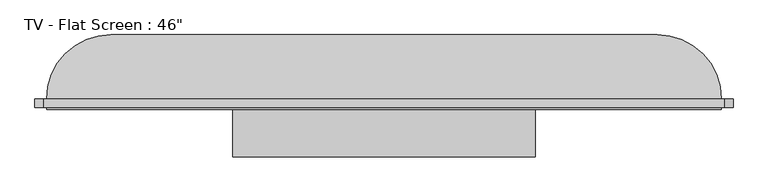
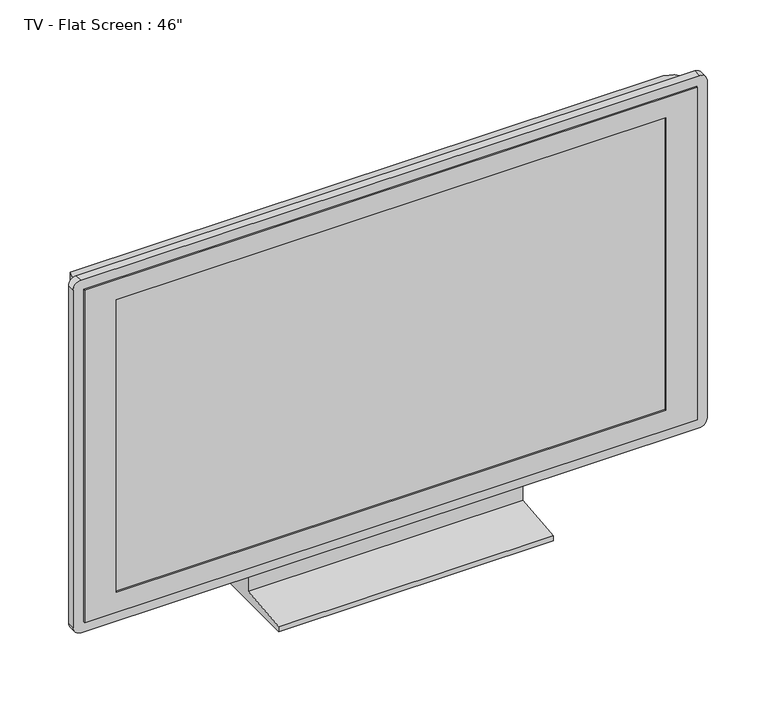
"""IFC4 building model written with IfcOpenShell, lengths in millimetres: furniture geometry."""

from ifc_helpers import new_model, si_unit, point, frame, frame_2d, origin, place, context, project, spatial, polyline, circle_curve, ellipse_curve, trimmed, segment, composite_curve, outline, extrude, faceted_brep, source, transform, mapped, element, save
from ifc_brep_helpers import plane_surface, cylinder_surface, advanced_brep


def furniture_d9bcc661(model_context):
    return source(origin(), model_context, "Body", "SolidModel", [
        extrude(outline(polyline([(-51.4613764, 80.0), (-1.4613764, 80.0), (48.5386236, 0.0), (-151.4613764, 0.0), (-151.4613764, 10.0), (-51.4613764, 20.0), (-51.4613764, 80.0)])), frame((-263.2325176, 0.0, 0.0), z_axis=(1.0, 0.0, 0.0), x_axis=(0.0, 1.0, 0.0)), (0.0, 0.0, 1.0), 518.576007),
        faceted_brep([(574.6314928, -69.4613764, 743.4515403), (-582.5205211, -69.4613764, 743.4515403), (-582.5205211, -69.4613764, 80.0), (574.6314928, -69.4613764, 80.0), (-522.5205211, -69.4613764, 703.4515403), (514.6314928, -69.4613764, 703.4515403), (514.6314928, -69.4613764, 120.0), (-522.5205211, -69.4613764, 120.0), (574.6314928, -51.4613764, 743.4515403), (574.6314928, -51.4613764, 80.0), (-582.5205211, -51.4613764, 80.0), (-582.5205211, -51.4613764, 743.4515403), (-522.5205211, -66.4613764, 703.4515403), (-522.5205211, -66.4613764, 120.0), (514.6314928, -66.4613764, 120.0), (514.6314928, -66.4613764, 703.4515403)], [[[0, 1, 2, 3], [4, 5, 6, 7]], [[8, 9, 10, 11]], [[1, 0, 8, 11]], [[2, 1, 11, 10]], [[3, 2, 10, 9]], [[0, 3, 9, 8]], [[12, 13, 14, 15]], [[12, 15, 5, 4]], [[15, 14, 6, 5]], [[14, 13, 7, 6]], [[13, 12, 4, 7]]]),
        extrude(outline(composite_curve([segment(polyline([(763.4515403, 579.6314928), (763.4515403, -587.5205211)]), True, "CONTINUOUS"), segment(trimmed(circle_curve(frame_2d((748.4515403, -587.5205211)), 15.0), [point((763.4515403, -587.5205211))], [point((748.4515403, -602.5205211))], False, "CARTESIAN"), True, "CONTINUOUS"), segment(polyline([(748.4515403, -602.5205211), (75.0, -602.5205211)]), True, "CONTINUOUS"), segment(trimmed(circle_curve(frame_2d((75.0, -587.5205211)), 15.0), [point((75.0, -602.5205211))], [point((60.0, -587.5205211))], False, "CARTESIAN"), True, "CONTINUOUS"), segment(polyline([(60.0, -587.5205211), (60.0, 579.6314928)]), True, "CONTINUOUS"), segment(trimmed(circle_curve(frame_2d((75.0, 579.6314928)), 15.0), [point((60.0, 579.6314928))], [point((75.0, 594.6314928))], False, "CARTESIAN"), True, "CONTINUOUS"), segment(polyline([(75.0, 594.6314928), (748.4515403, 594.6314928)]), True, "CONTINUOUS"), segment(trimmed(circle_curve(frame_2d((748.4515403, 579.6314928)), 15.0), [point((748.4515403, 594.6314928))], [point((763.4515403, 579.6314928))], False, "CARTESIAN"), True, "CONTINUOUS")], self_intersect=False), holes=[polyline([(743.4515403, 574.6314928), (80.0, 574.6314928), (80.0, -582.5205211), (743.4515403, -582.5205211), (743.4515403, 574.6314928)])]), frame((0.0, -66.4613764, 0.0), z_axis=(0.0, 1.0, 0.0), x_axis=(0.0, 0.0, 1.0)), (0.0, 0.0, 1.0), 15.0),
        advanced_brep(
        [(-582.5205211, -51.4613764, 80.0), (574.6314928, -51.4613764, 80.0), (574.6314928, -51.4613764, 743.4515403), (-582.5205211, -51.4613764, 743.4515403), (464.6314928, 58.5386236, 80.0), (-472.5205211, 58.5386236, 80.0), (-472.5205211, 58.5386236, 633.4515403), (464.6314928, 58.5386236, 633.4515403)],
        [
            (0, 1),
            (1, 2),
            (2, 3),
            (3, 0),
            (4, 5),
            (5, 6),
            (6, 7),
            (7, 4),
            (0, 5, circle_curve(frame((-472.5205211, -51.4613764, 80.0), z_axis=(0.0, 0.0, -1.0), x_axis=(-1.0, 0.0, 0.0)), 110.0)),
            (4, 1, circle_curve(frame((464.6314928, -51.4613764, 80.0), z_axis=(0.0, 0.0, -1.0), x_axis=(1.0, 0.0, 0.0)), 110.0)),
            (7, 2, ellipse_curve(frame((464.6314928, -51.4613764, 633.4515403), z_axis=(0.7071067811865475, 0.0, -0.7071067811865475), x_axis=(0.7071067811865474, 0.0, 0.7071067811865476)), 155.5634919, 110.0)),
            (6, 3, ellipse_curve(frame((-472.5205211, -51.4613764, 633.4515403), z_axis=(0.7071067811865475, 0.0, 0.7071067811865476), x_axis=(-0.7071067811865476, 0.0, 0.7071067811865475)), 155.5634919, 110.0)),
        ],
        [
            plane_surface(frame((-582.5205211, -51.4613764, 743.4515403), z_axis=(0.0, -1.0, 0.0), x_axis=(-1.0, 0.0, 0.0))),
            plane_surface(frame((-582.5205211, 58.5386236, 743.4515403), z_axis=(0.0, 1.0, 0.0), x_axis=(1.0, 0.0, 0.0))),
            plane_surface(frame((-582.5205211, -51.4613764, 80.0), z_axis=(0.0, 0.0, -1.0), x_axis=(0.0, 1.0, 0.0))),
            cylinder_surface(frame((464.6314928, -51.4613764, 80.0), z_axis=(0.0, 0.0, 1.0), x_axis=(1.0, 0.0, 0.0)), 110.0),
            cylinder_surface(frame((574.6314928, -51.4613764, 633.4515403), z_axis=(-1.0, 0.0, 0.0), x_axis=(0.0, 0.0, 1.0)), 110.0),
            cylinder_surface(frame((-472.5205211, -51.4613764, 743.4515403), z_axis=(0.0, 0.0, -1.0), x_axis=(-1.0, 0.0, 0.0)), 110.0),
        ],
        [
            (0, [[1, 2, 3, 4]]),
            (1, [[5, 6, 7, 8]]),
            (2, [[-1, 9, -5, 10]]),
            (3, [[11, -2, -10, -8]]),
            (4, [[-11, -7, 12, -3]]),
            (5, [[-12, -6, -9, -4]]),
        ],
    ),
    ])


if __name__ == "__main__":
    model = new_model("IFC4")
    model_context = context("Model", 3, world=origin())
    ifc_project = project(units=[si_unit("LENGTHUNIT", "METRE", prefix="MILLI")], contexts=[model_context])
    site = spatial("IfcSite", under=ifc_project)
    building = spatial("IfcBuilding", under=site)
    placement = place(None, origin())
    furniture_shape = furniture_d9bcc661(model_context)
    element("IfcFurniture", 1, ObjectType="TV - Flat Screen : 46\"", at=placement, inside=building, context=model_context, shape_type="MappedRepresentation", body=[
        mapped(furniture_shape, transform((0.0, 0.0, 0.0), x_axis=(1.0, 0.0, 0.0), y_axis=(0.0, 1.0, 0.0), z_axis=(0.0, 0.0, 1.0))),
    ])
    save(model, "model.ifc")

# Revit data of these elements
# Type "TV - Flat Screen : 46\""
#   SinAng = 0' - 0.0193"
#   L = 3' - 4.83276"
#   H = 1' - 10.97053"
#   Thickness = 0' - 4.33071"
#   Diagonal = 3' - 10.85039"
#   CosAng = 0' - 0.03431"
#   Stand [instance default] = yes
#   Default Elevation = 0
# Element 1 (IfcFurniture, "TV - Flat Screen : 46\"")
#   Materials on its faces: "TV - Black", "TV - Glass", "TV - Screen"
# Materials
#   "TV - Black": colour RGB 49 49 49, transparency 0
#   "TV - Glass": colour RGB 157 157 157, transparency 0.9
#   "TV - Screen": colour RGB 0 0 0, transparency 0
